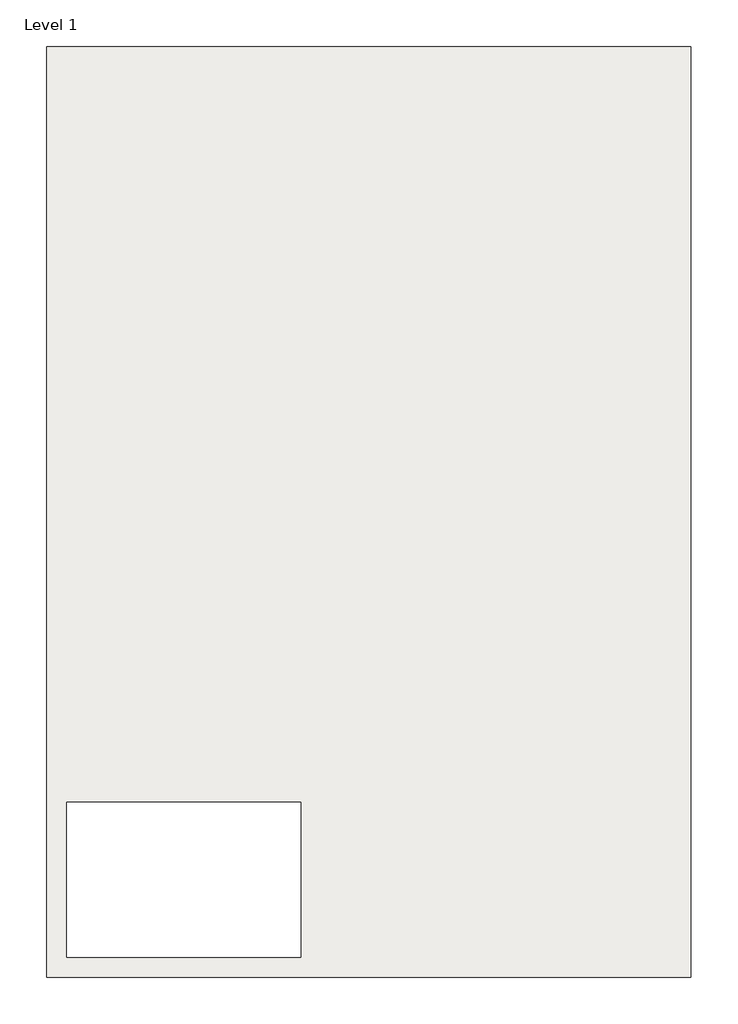
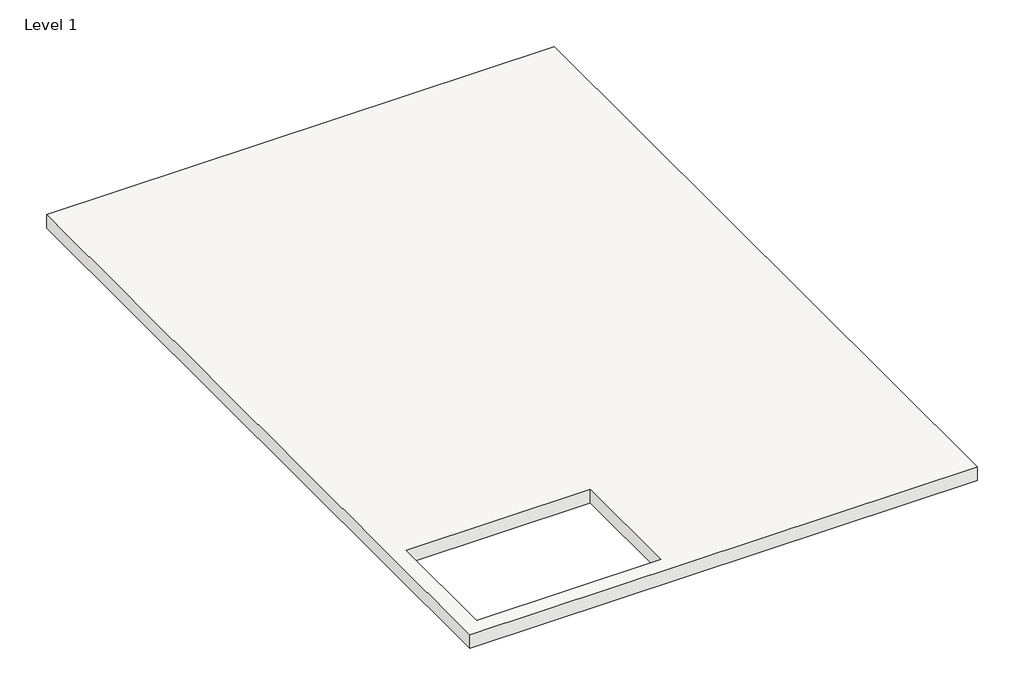
# One storey: 1 covering, 1 slab.
"""IFC4 building model written with IfcOpenShell, lengths in millimetres."""

from ifc_helpers import new_model, si_unit, frame, origin, place, context, project, spatial, polyline, outline, extrude, element, save

model = new_model("IFC4")

# Units and contexts
model_context = context("Model", 3, world=origin())
ifc_project = project(units=[si_unit("LENGTHUNIT", "METRE", prefix="MILLI")], contexts=[model_context])

# Site, building, storey
site = spatial("IfcSite", under=ifc_project)
building = spatial("IfcBuilding", under=site)
storey = spatial("IfcBuildingStorey", under=building, Name="Level 1", Elevation=3000.0)

# Covering
placement = place(None, origin())
element("IfcCovering", 1, ObjectType="Plain", at=placement, inside=storey, context=model_context, shape_type="SweptSolid", body=[
    extrude(outline(polyline([(-744.8904087, 11912.7642586), (-744.8904087, 2686.998858), (-744.8904087, 572.7642586), (-3784.8904087, 572.7642586), (-3784.8904087, 2686.998858), (-8434.8904087, 2686.998858), (-8434.8904087, 11912.7642586), (-744.8904087, 11912.7642586)])), frame((0.0, 0.0, 2600.0), z_axis=(0.0, 0.0, 1.0), x_axis=(1.0, 0.0, 0.0)), (0.0, 0.0, 1.0), 57.0),
])

# Slab
element("IfcSlab", 2, ObjectType="SLAB", at=placement, inside=storey, context=model_context, shape_type="SweptSolid", body=[
    extrude(outline(polyline([(-484.8904087, 12172.7642586), (-484.8904087, 312.7642586), (-8694.8904087, 312.7642586), (-8694.8904087, 12172.7642586), (-484.8904087, 12172.7642586)]), holes=[polyline([(-8434.8904087, 2546.998858), (-8434.8904087, 572.7642586), (-5458.9951322, 572.7642586), (-5458.9951322, 2546.998858), (-8434.8904087, 2546.998858)])]), frame((0.0, 0.0, 2570.0), z_axis=(0.0, 0.0, 1.0), x_axis=(1.0, 0.0, 0.0)), (0.0, 0.0, 1.0), 230.0),
])

save(model, "model.ifc")

# Revit data of these elements
# Type "Plain"
#   Keynote = "K40"
#   built-in parameter 1002203 = 1 (stored number, unit not read)
#   built-in parameter 1002202 = 1 (stored number, unit not read)
#   Layers, outside or top first: 45 mm "Metal Stud Layer" (function 1); 12 mm "Gypsum Wall Board" (function 1)
# Type "SLAB"
#   Layers, outside or top first: 230 mm no material (function 1)
# Element 1 (IfcCovering, "Plain")
#   Height Offset From Level = -400 mm
#   Phase Created = New Construction
#   Materials on its faces: "Gypsum Wall Board", "Metal Stud Layer"
# Element 2 (IfcSlab, "SLAB")
#   Height Offset From Level = -200 mm
#   built-in parameter 1001954 = 1
#   Phase Created = New Construction
# Materials
#   "Metal Stud Layer": class "Metal", colour RGB 127 127 127, transparency 0, Description = "Light gauge steel framing, thermal air layer", Cost = 0
#   "Gypsum Wall Board": class "Generic", colour RGB 249 249 249, transparency 0, Description = "Gypsum Wall Board", Cost = 0
